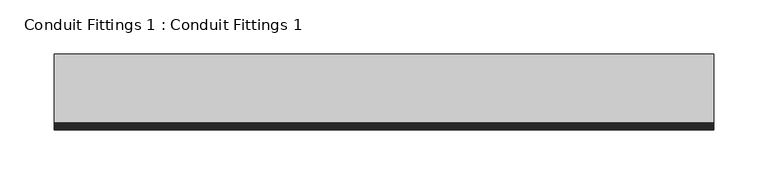
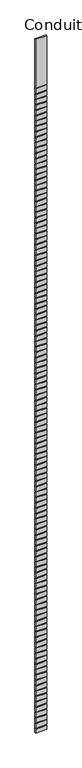
"""IFC4 building model written with IfcOpenShell, lengths in millimetres: cable carrier fitting geometry, Conduit Fittings 1 : Conduit Fittings 1."""

from ifc_helpers import new_model, si_unit, frame, origin, place, context, project, spatial, polyline, outline, extrude, source, transform, mapped, element, save


def conduit_fittings_1_conduit_fittings_1_d54f14cf(model_context):
    return source(origin(), model_context, "Body", "SweptSolid", [
        extrude(outline(polyline([(-5870.497125, -371.2934478), (-6480.097125, -371.2934478), (-6480.097125, -307.7934478), (-5870.497125, -307.7934478), (-5870.497125, -371.2934478)])), frame((0.0, 0.0, 2946.4), z_axis=(0.0, 0.0, 1.0), x_axis=(1.0, 0.0, 0.0)), (0.0, 0.0, 1.0), 225.4745322),
        extrude(outline(polyline([(-5870.497125, -371.2934478), (-6480.097125, -371.2934478), (-6480.097125, -307.7934478), (-5870.497125, -307.7934478), (-5870.497125, -371.2934478)])), frame((0.0, 0.0, 39493.8745322), z_axis=(0.0, 0.0, 1.0), x_axis=(1.0, 0.0, 0.0)), (0.0, 0.0, 1.0), 2771.7254678),
        extrude(outline(polyline([(-5870.497125, -371.2934478), (-6480.097125, -371.2934478), (-6480.097125, -307.7934478), (-5870.497125, -307.7934478), (-5870.497125, -371.2934478)])), frame((0.0, 0.0, 3222.6745322), z_axis=(0.0, 0.0, 1.0), x_axis=(1.0, 0.0, 0.0)), (0.0, 0.0, 1.0), 254.0),
        extrude(outline(polyline([(-5870.497125, -371.2934478), (-6480.097125, -371.2934478), (-6480.097125, -307.7934478), (-5870.497125, -307.7934478), (-5870.497125, -371.2934478)])), frame((0.0, 0.0, 3527.4745322), z_axis=(0.0, 0.0, 1.0), x_axis=(1.0, 0.0, 0.0)), (0.0, 0.0, 1.0), 254.0),
        extrude(outline(polyline([(-5870.497125, -371.2934478), (-6480.097125, -371.2934478), (-6480.097125, -307.7934478), (-5870.497125, -307.7934478), (-5870.497125, -371.2934478)])), frame((0.0, 0.0, 3832.2745322), z_axis=(0.0, 0.0, 1.0), x_axis=(1.0, 0.0, 0.0)), (0.0, 0.0, 1.0), 254.0),
        extrude(outline(polyline([(-5870.497125, -371.2934478), (-6480.097125, -371.2934478), (-6480.097125, -307.7934478), (-5870.497125, -307.7934478), (-5870.497125, -371.2934478)])), frame((0.0, 0.0, 4137.0745322), z_axis=(0.0, 0.0, 1.0), x_axis=(1.0, 0.0, 0.0)), (0.0, 0.0, 1.0), 254.0),
        extrude(outline(polyline([(-5870.497125, -371.2934478), (-6480.097125, -371.2934478), (-6480.097125, -307.7934478), (-5870.497125, -307.7934478), (-5870.497125, -371.2934478)])), frame((0.0, 0.0, 4441.8745322), z_axis=(0.0, 0.0, 1.0), x_axis=(1.0, 0.0, 0.0)), (0.0, 0.0, 1.0), 254.0),
        extrude(outline(polyline([(-5870.497125, -371.2934478), (-6480.097125, -371.2934478), (-6480.097125, -307.7934478), (-5870.497125, -307.7934478), (-5870.497125, -371.2934478)])), frame((0.0, 0.0, 4746.6745322), z_axis=(0.0, 0.0, 1.0), x_axis=(1.0, 0.0, 0.0)), (0.0, 0.0, 1.0), 254.0),
        extrude(outline(polyline([(-5870.497125, -371.2934478), (-6480.097125, -371.2934478), (-6480.097125, -307.7934478), (-5870.497125, -307.7934478), (-5870.497125, -371.2934478)])), frame((0.0, 0.0, 5051.4745322), z_axis=(0.0, 0.0, 1.0), x_axis=(1.0, 0.0, 0.0)), (0.0, 0.0, 1.0), 254.0),
        extrude(outline(polyline([(-5870.497125, -371.2934478), (-6480.097125, -371.2934478), (-6480.097125, -307.7934478), (-5870.497125, -307.7934478), (-5870.497125, -371.2934478)])), frame((0.0, 0.0, 5356.2745322), z_axis=(0.0, 0.0, 1.0), x_axis=(1.0, 0.0, 0.0)), (0.0, 0.0, 1.0), 254.0),
        extrude(outline(polyline([(-5870.497125, -371.2934478), (-6480.097125, -371.2934478), (-6480.097125, -307.7934478), (-5870.497125, -307.7934478), (-5870.497125, -371.2934478)])), frame((0.0, 0.0, 5661.0745322), z_axis=(0.0, 0.0, 1.0), x_axis=(1.0, 0.0, 0.0)), (0.0, 0.0, 1.0), 254.0),
        extrude(outline(polyline([(-5870.497125, -371.2934478), (-6480.097125, -371.2934478), (-6480.097125, -307.7934478), (-5870.497125, -307.7934478), (-5870.497125, -371.2934478)])), frame((0.0, 0.0, 5965.8745322), z_axis=(0.0, 0.0, 1.0), x_axis=(1.0, 0.0, 0.0)), (0.0, 0.0, 1.0), 254.0),
        extrude(outline(polyline([(-5870.497125, -371.2934478), (-6480.097125, -371.2934478), (-6480.097125, -307.7934478), (-5870.497125, -307.7934478), (-5870.497125, -371.2934478)])), frame((0.0, 0.0, 6270.6745322), z_axis=(0.0, 0.0, 1.0), x_axis=(1.0, 0.0, 0.0)), (0.0, 0.0, 1.0), 254.0),
        extrude(outline(polyline([(-5870.497125, -371.2934478), (-6480.097125, -371.2934478), (-6480.097125, -307.7934478), (-5870.497125, -307.7934478), (-5870.497125, -371.2934478)])), frame((0.0, 0.0, 6575.4745322), z_axis=(0.0, 0.0, 1.0), x_axis=(1.0, 0.0, 0.0)), (0.0, 0.0, 1.0), 254.0),
        extrude(outline(polyline([(-5870.497125, -371.2934478), (-6480.097125, -371.2934478), (-6480.097125, -307.7934478), (-5870.497125, -307.7934478), (-5870.497125, -371.2934478)])), frame((0.0, 0.0, 6880.2745322), z_axis=(0.0, 0.0, 1.0), x_axis=(1.0, 0.0, 0.0)), (0.0, 0.0, 1.0), 254.0),
        extrude(outline(polyline([(-5870.497125, -371.2934478), (-6480.097125, -371.2934478), (-6480.097125, -307.7934478), (-5870.497125, -307.7934478), (-5870.497125, -371.2934478)])), frame((0.0, 0.0, 7185.0745322), z_axis=(0.0, 0.0, 1.0), x_axis=(1.0, 0.0, 0.0)), (0.0, 0.0, 1.0), 254.0),
        extrude(outline(polyline([(-5870.497125, -371.2934478), (-6480.097125, -371.2934478), (-6480.097125, -307.7934478), (-5870.497125, -307.7934478), (-5870.497125, -371.2934478)])), frame((0.0, 0.0, 7489.8745322), z_axis=(0.0, 0.0, 1.0), x_axis=(1.0, 0.0, 0.0)), (0.0, 0.0, 1.0), 254.0),
        extrude(outline(polyline([(-5870.497125, -371.2934478), (-6480.097125, -371.2934478), (-6480.097125, -307.7934478), (-5870.497125, -307.7934478), (-5870.497125, -371.2934478)])), frame((0.0, 0.0, 7794.6745322), z_axis=(0.0, 0.0, 1.0), x_axis=(1.0, 0.0, 0.0)), (0.0, 0.0, 1.0), 254.0),
        extrude(outline(polyline([(-5870.497125, -371.2934478), (-6480.097125, -371.2934478), (-6480.097125, -307.7934478), (-5870.497125, -307.7934478), (-5870.497125, -371.2934478)])), frame((0.0, 0.0, 8099.4745322), z_axis=(0.0, 0.0, 1.0), x_axis=(1.0, 0.0, 0.0)), (0.0, 0.0, 1.0), 254.0),
        extrude(outline(polyline([(-5870.497125, -371.2934478), (-6480.097125, -371.2934478), (-6480.097125, -307.7934478), (-5870.497125, -307.7934478), (-5870.497125, -371.2934478)])), frame((0.0, 0.0, 8404.2745322), z_axis=(0.0, 0.0, 1.0), x_axis=(1.0, 0.0, 0.0)), (0.0, 0.0, 1.0), 254.0),
        extrude(outline(polyline([(-5870.497125, -371.2934478), (-6480.097125, -371.2934478), (-6480.097125, -307.7934478), (-5870.497125, -307.7934478), (-5870.497125, -371.2934478)])), frame((0.0, 0.0, 8709.0745322), z_axis=(0.0, 0.0, 1.0), x_axis=(1.0, 0.0, 0.0)), (0.0, 0.0, 1.0), 254.0),
        extrude(outline(polyline([(-5870.497125, -371.2934478), (-6480.097125, -371.2934478), (-6480.097125, -307.7934478), (-5870.497125, -307.7934478), (-5870.497125, -371.2934478)])), frame((0.0, 0.0, 9013.8745322), z_axis=(0.0, 0.0, 1.0), x_axis=(1.0, 0.0, 0.0)), (0.0, 0.0, 1.0), 254.0),
        extrude(outline(polyline([(-5870.497125, -371.2934478), (-6480.097125, -371.2934478), (-6480.097125, -307.7934478), (-5870.497125, -307.7934478), (-5870.497125, -371.2934478)])), frame((0.0, 0.0, 9318.6745322), z_axis=(0.0, 0.0, 1.0), x_axis=(1.0, 0.0, 0.0)), (0.0, 0.0, 1.0), 254.0),
        extrude(outline(polyline([(-5870.497125, -371.2934478), (-6480.097125, -371.2934478), (-6480.097125, -307.7934478), (-5870.497125, -307.7934478), (-5870.497125, -371.2934478)])), frame((0.0, 0.0, 9623.4745322), z_axis=(0.0, 0.0, 1.0), x_axis=(1.0, 0.0, 0.0)), (0.0, 0.0, 1.0), 254.0),
        extrude(outline(polyline([(-5870.497125, -371.2934478), (-6480.097125, -371.2934478), (-6480.097125, -307.7934478), (-5870.497125, -307.7934478), (-5870.497125, -371.2934478)])), frame((0.0, 0.0, 9928.2745322), z_axis=(0.0, 0.0, 1.0), x_axis=(1.0, 0.0, 0.0)), (0.0, 0.0, 1.0), 254.0),
        extrude(outline(polyline([(-5870.497125, -371.2934478), (-6480.097125, -371.2934478), (-6480.097125, -307.7934478), (-5870.497125, -307.7934478), (-5870.497125, -371.2934478)])), frame((0.0, 0.0, 10233.0745322), z_axis=(0.0, 0.0, 1.0), x_axis=(1.0, 0.0, 0.0)), (0.0, 0.0, 1.0), 254.0),
        extrude(outline(polyline([(-5870.497125, -371.2934478), (-6480.097125, -371.2934478), (-6480.097125, -307.7934478), (-5870.497125, -307.7934478), (-5870.497125, -371.2934478)])), frame((0.0, 0.0, 10537.8745322), z_axis=(0.0, 0.0, 1.0), x_axis=(1.0, 0.0, 0.0)), (0.0, 0.0, 1.0), 254.0),
        extrude(outline(polyline([(-5870.497125, -371.2934478), (-6480.097125, -371.2934478), (-6480.097125, -307.7934478), (-5870.497125, -307.7934478), (-5870.497125, -371.2934478)])), frame((0.0, 0.0, 10842.6745322), z_axis=(0.0, 0.0, 1.0), x_axis=(1.0, 0.0, 0.0)), (0.0, 0.0, 1.0), 254.0),
        extrude(outline(polyline([(-5870.497125, -371.2934478), (-6480.097125, -371.2934478), (-6480.097125, -307.7934478), (-5870.497125, -307.7934478), (-5870.497125, -371.2934478)])), frame((0.0, 0.0, 11147.4745322), z_axis=(0.0, 0.0, 1.0), x_axis=(1.0, 0.0, 0.0)), (0.0, 0.0, 1.0), 254.0),
        extrude(outline(polyline([(-5870.497125, -371.2934478), (-6480.097125, -371.2934478), (-6480.097125, -307.7934478), (-5870.497125, -307.7934478), (-5870.497125, -371.2934478)])), frame((0.0, 0.0, 11452.2745322), z_axis=(0.0, 0.0, 1.0), x_axis=(1.0, 0.0, 0.0)), (0.0, 0.0, 1.0), 254.0),
        extrude(outline(polyline([(-5870.497125, -371.2934478), (-6480.097125, -371.2934478), (-6480.097125, -307.7934478), (-5870.497125, -307.7934478), (-5870.497125, -371.2934478)])), frame((0.0, 0.0, 11757.0745322), z_axis=(0.0, 0.0, 1.0), x_axis=(1.0, 0.0, 0.0)), (0.0, 0.0, 1.0), 254.0),
        extrude(outline(polyline([(-5870.497125, -371.2934478), (-6480.097125, -371.2934478), (-6480.097125, -307.7934478), (-5870.497125, -307.7934478), (-5870.497125, -371.2934478)])), frame((0.0, 0.0, 12061.8745322), z_axis=(0.0, 0.0, 1.0), x_axis=(1.0, 0.0, 0.0)), (0.0, 0.0, 1.0), 254.0),
        extrude(outline(polyline([(-5870.497125, -371.2934478), (-6480.097125, -371.2934478), (-6480.097125, -307.7934478), (-5870.497125, -307.7934478), (-5870.497125, -371.2934478)])), frame((0.0, 0.0, 12366.6745322), z_axis=(0.0, 0.0, 1.0), x_axis=(1.0, 0.0, 0.0)), (0.0, 0.0, 1.0), 254.0),
        extrude(outline(polyline([(-5870.497125, -371.2934478), (-6480.097125, -371.2934478), (-6480.097125, -307.7934478), (-5870.497125, -307.7934478), (-5870.497125, -371.2934478)])), frame((0.0, 0.0, 12671.4745322), z_axis=(0.0, 0.0, 1.0), x_axis=(1.0, 0.0, 0.0)), (0.0, 0.0, 1.0), 254.0),
        extrude(outline(polyline([(-5870.497125, -371.2934478), (-6480.097125, -371.2934478), (-6480.097125, -307.7934478), (-5870.497125, -307.7934478), (-5870.497125, -371.2934478)])), frame((0.0, 0.0, 12976.2745322), z_axis=(0.0, 0.0, 1.0), x_axis=(1.0, 0.0, 0.0)), (0.0, 0.0, 1.0), 254.0),
        extrude(outline(polyline([(-5870.497125, -371.2934478), (-6480.097125, -371.2934478), (-6480.097125, -307.7934478), (-5870.497125, -307.7934478), (-5870.497125, -371.2934478)])), frame((0.0, 0.0, 13281.0745322), z_axis=(0.0, 0.0, 1.0), x_axis=(1.0, 0.0, 0.0)), (0.0, 0.0, 1.0), 254.0),
        extrude(outline(polyline([(-5870.497125, -371.2934478), (-6480.097125, -371.2934478), (-6480.097125, -307.7934478), (-5870.497125, -307.7934478), (-5870.497125, -371.2934478)])), frame((0.0, 0.0, 13585.8745322), z_axis=(0.0, 0.0, 1.0), x_axis=(1.0, 0.0, 0.0)), (0.0, 0.0, 1.0), 254.0),
        extrude(outline(polyline([(-5870.497125, -371.2934478), (-6480.097125, -371.2934478), (-6480.097125, -307.7934478), (-5870.497125, -307.7934478), (-5870.497125, -371.2934478)])), frame((0.0, 0.0, 13890.6745322), z_axis=(0.0, 0.0, 1.0), x_axis=(1.0, 0.0, 0.0)), (0.0, 0.0, 1.0), 254.0),
        extrude(outline(polyline([(-5870.497125, -371.2934478), (-6480.097125, -371.2934478), (-6480.097125, -307.7934478), (-5870.497125, -307.7934478), (-5870.497125, -371.2934478)])), frame((0.0, 0.0, 14195.4745322), z_axis=(0.0, 0.0, 1.0), x_axis=(1.0, 0.0, 0.0)), (0.0, 0.0, 1.0), 254.0),
        extrude(outline(polyline([(-5870.497125, -371.2934478), (-6480.097125, -371.2934478), (-6480.097125, -307.7934478), (-5870.497125, -307.7934478), (-5870.497125, -371.2934478)])), frame((0.0, 0.0, 14500.2745322), z_axis=(0.0, 0.0, 1.0), x_axis=(1.0, 0.0, 0.0)), (0.0, 0.0, 1.0), 254.0),
        extrude(outline(polyline([(-5870.497125, -371.2934478), (-6480.097125, -371.2934478), (-6480.097125, -307.7934478), (-5870.497125, -307.7934478), (-5870.497125, -371.2934478)])), frame((0.0, 0.0, 14805.0745322), z_axis=(0.0, 0.0, 1.0), x_axis=(1.0, 0.0, 0.0)), (0.0, 0.0, 1.0), 254.0),
        extrude(outline(polyline([(-5870.497125, -371.2934478), (-6480.097125, -371.2934478), (-6480.097125, -307.7934478), (-5870.497125, -307.7934478), (-5870.497125, -371.2934478)])), frame((0.0, 0.0, 15109.8745322), z_axis=(0.0, 0.0, 1.0), x_axis=(1.0, 0.0, 0.0)), (0.0, 0.0, 1.0), 254.0),
        extrude(outline(polyline([(-5870.497125, -371.2934478), (-6480.097125, -371.2934478), (-6480.097125, -307.7934478), (-5870.497125, -307.7934478), (-5870.497125, -371.2934478)])), frame((0.0, 0.0, 15414.6745322), z_axis=(0.0, 0.0, 1.0), x_axis=(1.0, 0.0, 0.0)), (0.0, 0.0, 1.0), 254.0),
        extrude(outline(polyline([(-5870.497125, -371.2934478), (-6480.097125, -371.2934478), (-6480.097125, -307.7934478), (-5870.497125, -307.7934478), (-5870.497125, -371.2934478)])), frame((0.0, 0.0, 15719.4745322), z_axis=(0.0, 0.0, 1.0), x_axis=(1.0, 0.0, 0.0)), (0.0, 0.0, 1.0), 254.0),
        extrude(outline(polyline([(-5870.497125, -371.2934478), (-6480.097125, -371.2934478), (-6480.097125, -307.7934478), (-5870.497125, -307.7934478), (-5870.497125, -371.2934478)])), frame((0.0, 0.0, 16024.2745322), z_axis=(0.0, 0.0, 1.0), x_axis=(1.0, 0.0, 0.0)), (0.0, 0.0, 1.0), 254.0),
        extrude(outline(polyline([(-5870.497125, -371.2934478), (-6480.097125, -371.2934478), (-6480.097125, -307.7934478), (-5870.497125, -307.7934478), (-5870.497125, -371.2934478)])), frame((0.0, 0.0, 16329.0745322), z_axis=(0.0, 0.0, 1.0), x_axis=(1.0, 0.0, 0.0)), (0.0, 0.0, 1.0), 254.0),
        extrude(outline(polyline([(-5870.497125, -371.2934478), (-6480.097125, -371.2934478), (-6480.097125, -307.7934478), (-5870.497125, -307.7934478), (-5870.497125, -371.2934478)])), frame((0.0, 0.0, 16633.8745322), z_axis=(0.0, 0.0, 1.0), x_axis=(1.0, 0.0, 0.0)), (0.0, 0.0, 1.0), 254.0),
        extrude(outline(polyline([(-5870.497125, -371.2934478), (-6480.097125, -371.2934478), (-6480.097125, -307.7934478), (-5870.497125, -307.7934478), (-5870.497125, -371.2934478)])), frame((0.0, 0.0, 16938.6745322), z_axis=(0.0, 0.0, 1.0), x_axis=(1.0, 0.0, 0.0)), (0.0, 0.0, 1.0), 254.0),
        extrude(outline(polyline([(-5870.497125, -371.2934478), (-6480.097125, -371.2934478), (-6480.097125, -307.7934478), (-5870.497125, -307.7934478), (-5870.497125, -371.2934478)])), frame((0.0, 0.0, 17243.4745322), z_axis=(0.0, 0.0, 1.0), x_axis=(1.0, 0.0, 0.0)), (0.0, 0.0, 1.0), 254.0),
        extrude(outline(polyline([(-5870.497125, -371.2934478), (-6480.097125, -371.2934478), (-6480.097125, -307.7934478), (-5870.497125, -307.7934478), (-5870.497125, -371.2934478)])), frame((0.0, 0.0, 17548.2745322), z_axis=(0.0, 0.0, 1.0), x_axis=(1.0, 0.0, 0.0)), (0.0, 0.0, 1.0), 254.0),
        extrude(outline(polyline([(-5870.497125, -371.2934478), (-6480.097125, -371.2934478), (-6480.097125, -307.7934478), (-5870.497125, -307.7934478), (-5870.497125, -371.2934478)])), frame((0.0, 0.0, 17853.0745322), z_axis=(0.0, 0.0, 1.0), x_axis=(1.0, 0.0, 0.0)), (0.0, 0.0, 1.0), 254.0),
        extrude(outline(polyline([(-5870.497125, -371.2934478), (-6480.097125, -371.2934478), (-6480.097125, -307.7934478), (-5870.497125, -307.7934478), (-5870.497125, -371.2934478)])), frame((0.0, 0.0, 18157.8745322), z_axis=(0.0, 0.0, 1.0), x_axis=(1.0, 0.0, 0.0)), (0.0, 0.0, 1.0), 254.0),
        extrude(outline(polyline([(-5870.497125, -371.2934478), (-6480.097125, -371.2934478), (-6480.097125, -307.7934478), (-5870.497125, -307.7934478), (-5870.497125, -371.2934478)])), frame((0.0, 0.0, 18462.6745322), z_axis=(0.0, 0.0, 1.0), x_axis=(1.0, 0.0, 0.0)), (0.0, 0.0, 1.0), 254.0),
        extrude(outline(polyline([(-5870.497125, -371.2934478), (-6480.097125, -371.2934478), (-6480.097125, -307.7934478), (-5870.497125, -307.7934478), (-5870.497125, -371.2934478)])), frame((0.0, 0.0, 18767.4745322), z_axis=(0.0, 0.0, 1.0), x_axis=(1.0, 0.0, 0.0)), (0.0, 0.0, 1.0), 254.0),
        extrude(outline(polyline([(-5870.497125, -371.2934478), (-6480.097125, -371.2934478), (-6480.097125, -307.7934478), (-5870.497125, -307.7934478), (-5870.497125, -371.2934478)])), frame((0.0, 0.0, 19072.2745322), z_axis=(0.0, 0.0, 1.0), x_axis=(1.0, 0.0, 0.0)), (0.0, 0.0, 1.0), 254.0),
        extrude(outline(polyline([(-5870.497125, -371.2934478), (-6480.097125, -371.2934478), (-6480.097125, -307.7934478), (-5870.497125, -307.7934478), (-5870.497125, -371.2934478)])), frame((0.0, 0.0, 19377.0745322), z_axis=(0.0, 0.0, 1.0), x_axis=(1.0, 0.0, 0.0)), (0.0, 0.0, 1.0), 254.0),
        extrude(outline(polyline([(-5870.497125, -371.2934478), (-6480.097125, -371.2934478), (-6480.097125, -307.7934478), (-5870.497125, -307.7934478), (-5870.497125, -371.2934478)])), frame((0.0, 0.0, 19681.8745322), z_axis=(0.0, 0.0, 1.0), x_axis=(1.0, 0.0, 0.0)), (0.0, 0.0, 1.0), 254.0),
        extrude(outline(polyline([(-5870.497125, -371.2934478), (-6480.097125, -371.2934478), (-6480.097125, -307.7934478), (-5870.497125, -307.7934478), (-5870.497125, -371.2934478)])), frame((0.0, 0.0, 19986.6745322), z_axis=(0.0, 0.0, 1.0), x_axis=(1.0, 0.0, 0.0)), (0.0, 0.0, 1.0), 254.0),
        extrude(outline(polyline([(-5870.497125, -371.2934478), (-6480.097125, -371.2934478), (-6480.097125, -307.7934478), (-5870.497125, -307.7934478), (-5870.497125, -371.2934478)])), frame((0.0, 0.0, 20291.4745322), z_axis=(0.0, 0.0, 1.0), x_axis=(1.0, 0.0, 0.0)), (0.0, 0.0, 1.0), 254.0),
        extrude(outline(polyline([(-5870.497125, -371.2934478), (-6480.097125, -371.2934478), (-6480.097125, -307.7934478), (-5870.497125, -307.7934478), (-5870.497125, -371.2934478)])), frame((0.0, 0.0, 20596.2745322), z_axis=(0.0, 0.0, 1.0), x_axis=(1.0, 0.0, 0.0)), (0.0, 0.0, 1.0), 254.0),
        extrude(outline(polyline([(-5870.497125, -371.2934478), (-6480.097125, -371.2934478), (-6480.097125, -307.7934478), (-5870.497125, -307.7934478), (-5870.497125, -371.2934478)])), frame((0.0, 0.0, 20901.0745322), z_axis=(0.0, 0.0, 1.0), x_axis=(1.0, 0.0, 0.0)), (0.0, 0.0, 1.0), 254.0),
        extrude(outline(polyline([(-5870.497125, -371.2934478), (-6480.097125, -371.2934478), (-6480.097125, -307.7934478), (-5870.497125, -307.7934478), (-5870.497125, -371.2934478)])), frame((0.0, 0.0, 21205.8745322), z_axis=(0.0, 0.0, 1.0), x_axis=(1.0, 0.0, 0.0)), (0.0, 0.0, 1.0), 254.0),
        extrude(outline(polyline([(-5870.497125, -371.2934478), (-6480.097125, -371.2934478), (-6480.097125, -307.7934478), (-5870.497125, -307.7934478), (-5870.497125, -371.2934478)])), frame((0.0, 0.0, 21510.6745322), z_axis=(0.0, 0.0, 1.0), x_axis=(1.0, 0.0, 0.0)), (0.0, 0.0, 1.0), 254.0),
        extrude(outline(polyline([(-5870.497125, -371.2934478), (-6480.097125, -371.2934478), (-6480.097125, -307.7934478), (-5870.497125, -307.7934478), (-5870.497125, -371.2934478)])), frame((0.0, 0.0, 21815.4745322), z_axis=(0.0, 0.0, 1.0), x_axis=(1.0, 0.0, 0.0)), (0.0, 0.0, 1.0), 254.0),
        extrude(outline(polyline([(-5870.497125, -371.2934478), (-6480.097125, -371.2934478), (-6480.097125, -307.7934478), (-5870.497125, -307.7934478), (-5870.497125, -371.2934478)])), frame((0.0, 0.0, 22120.2745322), z_axis=(0.0, 0.0, 1.0), x_axis=(1.0, 0.0, 0.0)), (0.0, 0.0, 1.0), 254.0),
        extrude(outline(polyline([(-5870.497125, -371.2934478), (-6480.097125, -371.2934478), (-6480.097125, -307.7934478), (-5870.497125, -307.7934478), (-5870.497125, -371.2934478)])), frame((0.0, 0.0, 22425.0745322), z_axis=(0.0, 0.0, 1.0), x_axis=(1.0, 0.0, 0.0)), (0.0, 0.0, 1.0), 254.0),
        extrude(outline(polyline([(-5870.497125, -371.2934478), (-6480.097125, -371.2934478), (-6480.097125, -307.7934478), (-5870.497125, -307.7934478), (-5870.497125, -371.2934478)])), frame((0.0, 0.0, 22729.8745322), z_axis=(0.0, 0.0, 1.0), x_axis=(1.0, 0.0, 0.0)), (0.0, 0.0, 1.0), 254.0),
        extrude(outline(polyline([(-5870.497125, -371.2934478), (-6480.097125, -371.2934478), (-6480.097125, -307.7934478), (-5870.497125, -307.7934478), (-5870.497125, -371.2934478)])), frame((0.0, 0.0, 23034.6745322), z_axis=(0.0, 0.0, 1.0), x_axis=(1.0, 0.0, 0.0)), (0.0, 0.0, 1.0), 254.0),
        extrude(outline(polyline([(-5870.497125, -371.2934478), (-6480.097125, -371.2934478), (-6480.097125, -307.7934478), (-5870.497125, -307.7934478), (-5870.497125, -371.2934478)])), frame((0.0, 0.0, 23339.4745322), z_axis=(0.0, 0.0, 1.0), x_axis=(1.0, 0.0, 0.0)), (0.0, 0.0, 1.0), 254.0),
        extrude(outline(polyline([(-5870.497125, -371.2934478), (-6480.097125, -371.2934478), (-6480.097125, -307.7934478), (-5870.497125, -307.7934478), (-5870.497125, -371.2934478)])), frame((0.0, 0.0, 23644.2745322), z_axis=(0.0, 0.0, 1.0), x_axis=(1.0, 0.0, 0.0)), (0.0, 0.0, 1.0), 254.0),
        extrude(outline(polyline([(-5870.497125, -371.2934478), (-6480.097125, -371.2934478), (-6480.097125, -307.7934478), (-5870.497125, -307.7934478), (-5870.497125, -371.2934478)])), frame((0.0, 0.0, 23949.0745322), z_axis=(0.0, 0.0, 1.0), x_axis=(1.0, 0.0, 0.0)), (0.0, 0.0, 1.0), 254.0),
        extrude(outline(polyline([(-5870.497125, -371.2934478), (-6480.097125, -371.2934478), (-6480.097125, -307.7934478), (-5870.497125, -307.7934478), (-5870.497125, -371.2934478)])), frame((0.0, 0.0, 24253.8745322), z_axis=(0.0, 0.0, 1.0), x_axis=(1.0, 0.0, 0.0)), (0.0, 0.0, 1.0), 254.0),
        extrude(outline(polyline([(-5870.497125, -371.2934478), (-6480.097125, -371.2934478), (-6480.097125, -307.7934478), (-5870.497125, -307.7934478), (-5870.497125, -371.2934478)])), frame((0.0, 0.0, 24558.6745322), z_axis=(0.0, 0.0, 1.0), x_axis=(1.0, 0.0, 0.0)), (0.0, 0.0, 1.0), 254.0),
        extrude(outline(polyline([(-5870.497125, -371.2934478), (-6480.097125, -371.2934478), (-6480.097125, -307.7934478), (-5870.497125, -307.7934478), (-5870.497125, -371.2934478)])), frame((0.0, 0.0, 24863.4745322), z_axis=(0.0, 0.0, 1.0), x_axis=(1.0, 0.0, 0.0)), (0.0, 0.0, 1.0), 254.0),
        extrude(outline(polyline([(-5870.497125, -371.2934478), (-6480.097125, -371.2934478), (-6480.097125, -307.7934478), (-5870.497125, -307.7934478), (-5870.497125, -371.2934478)])), frame((0.0, 0.0, 25168.2745322), z_axis=(0.0, 0.0, 1.0), x_axis=(1.0, 0.0, 0.0)), (0.0, 0.0, 1.0), 254.0),
        extrude(outline(polyline([(-5870.497125, -371.2934478), (-6480.097125, -371.2934478), (-6480.097125, -307.7934478), (-5870.497125, -307.7934478), (-5870.497125, -371.2934478)])), frame((0.0, 0.0, 25473.0745322), z_axis=(0.0, 0.0, 1.0), x_axis=(1.0, 0.0, 0.0)), (0.0, 0.0, 1.0), 254.0),
        extrude(outline(polyline([(-5870.497125, -371.2934478), (-6480.097125, -371.2934478), (-6480.097125, -307.7934478), (-5870.497125, -307.7934478), (-5870.497125, -371.2934478)])), frame((0.0, 0.0, 25777.8745322), z_axis=(0.0, 0.0, 1.0), x_axis=(1.0, 0.0, 0.0)), (0.0, 0.0, 1.0), 254.0),
        extrude(outline(polyline([(-5870.497125, -371.2934478), (-6480.097125, -371.2934478), (-6480.097125, -307.7934478), (-5870.497125, -307.7934478), (-5870.497125, -371.2934478)])), frame((0.0, 0.0, 26082.6745322), z_axis=(0.0, 0.0, 1.0), x_axis=(1.0, 0.0, 0.0)), (0.0, 0.0, 1.0), 254.0),
        extrude(outline(polyline([(-5870.497125, -371.2934478), (-6480.097125, -371.2934478), (-6480.097125, -307.7934478), (-5870.497125, -307.7934478), (-5870.497125, -371.2934478)])), frame((0.0, 0.0, 26387.4745322), z_axis=(0.0, 0.0, 1.0), x_axis=(1.0, 0.0, 0.0)), (0.0, 0.0, 1.0), 254.0),
        extrude(outline(polyline([(-5870.497125, -371.2934478), (-6480.097125, -371.2934478), (-6480.097125, -307.7934478), (-5870.497125, -307.7934478), (-5870.497125, -371.2934478)])), frame((0.0, 0.0, 26692.2745322), z_axis=(0.0, 0.0, 1.0), x_axis=(1.0, 0.0, 0.0)), (0.0, 0.0, 1.0), 254.0),
        extrude(outline(polyline([(-5870.497125, -371.2934478), (-6480.097125, -371.2934478), (-6480.097125, -307.7934478), (-5870.497125, -307.7934478), (-5870.497125, -371.2934478)])), frame((0.0, 0.0, 26997.0745322), z_axis=(0.0, 0.0, 1.0), x_axis=(1.0, 0.0, 0.0)), (0.0, 0.0, 1.0), 254.0),
        extrude(outline(polyline([(-5870.497125, -371.2934478), (-6480.097125, -371.2934478), (-6480.097125, -307.7934478), (-5870.497125, -307.7934478), (-5870.497125, -371.2934478)])), frame((0.0, 0.0, 27301.8745322), z_axis=(0.0, 0.0, 1.0), x_axis=(1.0, 0.0, 0.0)), (0.0, 0.0, 1.0), 254.0),
        extrude(outline(polyline([(-5870.497125, -371.2934478), (-6480.097125, -371.2934478), (-6480.097125, -307.7934478), (-5870.497125, -307.7934478), (-5870.497125, -371.2934478)])), frame((0.0, 0.0, 27606.6745322), z_axis=(0.0, 0.0, 1.0), x_axis=(1.0, 0.0, 0.0)), (0.0, 0.0, 1.0), 254.0),
        extrude(outline(polyline([(-5870.497125, -371.2934478), (-6480.097125, -371.2934478), (-6480.097125, -307.7934478), (-5870.497125, -307.7934478), (-5870.497125, -371.2934478)])), frame((0.0, 0.0, 27911.4745322), z_axis=(0.0, 0.0, 1.0), x_axis=(1.0, 0.0, 0.0)), (0.0, 0.0, 1.0), 254.0),
        extrude(outline(polyline([(-5870.497125, -371.2934478), (-6480.097125, -371.2934478), (-6480.097125, -307.7934478), (-5870.497125, -307.7934478), (-5870.497125, -371.2934478)])), frame((0.0, 0.0, 28216.2745322), z_axis=(0.0, 0.0, 1.0), x_axis=(1.0, 0.0, 0.0)), (0.0, 0.0, 1.0), 254.0),
        extrude(outline(polyline([(-5870.497125, -371.2934478), (-6480.097125, -371.2934478), (-6480.097125, -307.7934478), (-5870.497125, -307.7934478), (-5870.497125, -371.2934478)])), frame((0.0, 0.0, 28521.0745322), z_axis=(0.0, 0.0, 1.0), x_axis=(1.0, 0.0, 0.0)), (0.0, 0.0, 1.0), 254.0),
        extrude(outline(polyline([(-5870.497125, -371.2934478), (-6480.097125, -371.2934478), (-6480.097125, -307.7934478), (-5870.497125, -307.7934478), (-5870.497125, -371.2934478)])), frame((0.0, 0.0, 28825.8745322), z_axis=(0.0, 0.0, 1.0), x_axis=(1.0, 0.0, 0.0)), (0.0, 0.0, 1.0), 254.0),
        extrude(outline(polyline([(-5870.497125, -371.2934478), (-6480.097125, -371.2934478), (-6480.097125, -307.7934478), (-5870.497125, -307.7934478), (-5870.497125, -371.2934478)])), frame((0.0, 0.0, 29130.6745322), z_axis=(0.0, 0.0, 1.0), x_axis=(1.0, 0.0, 0.0)), (0.0, 0.0, 1.0), 254.0),
        extrude(outline(polyline([(-5870.497125, -371.2934478), (-6480.097125, -371.2934478), (-6480.097125, -307.7934478), (-5870.497125, -307.7934478), (-5870.497125, -371.2934478)])), frame((0.0, 0.0, 29435.4745322), z_axis=(0.0, 0.0, 1.0), x_axis=(1.0, 0.0, 0.0)), (0.0, 0.0, 1.0), 254.0),
        extrude(outline(polyline([(-5870.497125, -371.2934478), (-6480.097125, -371.2934478), (-6480.097125, -307.7934478), (-5870.497125, -307.7934478), (-5870.497125, -371.2934478)])), frame((0.0, 0.0, 29740.2745322), z_axis=(0.0, 0.0, 1.0), x_axis=(1.0, 0.0, 0.0)), (0.0, 0.0, 1.0), 254.0),
        extrude(outline(polyline([(-5870.497125, -371.2934478), (-6480.097125, -371.2934478), (-6480.097125, -307.7934478), (-5870.497125, -307.7934478), (-5870.497125, -371.2934478)])), frame((0.0, 0.0, 30045.0745322), z_axis=(0.0, 0.0, 1.0), x_axis=(1.0, 0.0, 0.0)), (0.0, 0.0, 1.0), 254.0),
        extrude(outline(polyline([(-5870.497125, -371.2934478), (-6480.097125, -371.2934478), (-6480.097125, -307.7934478), (-5870.497125, -307.7934478), (-5870.497125, -371.2934478)])), frame((0.0, 0.0, 30349.8745322), z_axis=(0.0, 0.0, 1.0), x_axis=(1.0, 0.0, 0.0)), (0.0, 0.0, 1.0), 254.0),
        extrude(outline(polyline([(-5870.497125, -371.2934478), (-6480.097125, -371.2934478), (-6480.097125, -307.7934478), (-5870.497125, -307.7934478), (-5870.497125, -371.2934478)])), frame((0.0, 0.0, 30654.6745322), z_axis=(0.0, 0.0, 1.0), x_axis=(1.0, 0.0, 0.0)), (0.0, 0.0, 1.0), 254.0),
        extrude(outline(polyline([(-5870.497125, -371.2934478), (-6480.097125, -371.2934478), (-6480.097125, -307.7934478), (-5870.497125, -307.7934478), (-5870.497125, -371.2934478)])), frame((0.0, 0.0, 30959.4745322), z_axis=(0.0, 0.0, 1.0), x_axis=(1.0, 0.0, 0.0)), (0.0, 0.0, 1.0), 254.0),
        extrude(outline(polyline([(-5870.497125, -371.2934478), (-6480.097125, -371.2934478), (-6480.097125, -307.7934478), (-5870.497125, -307.7934478), (-5870.497125, -371.2934478)])), frame((0.0, 0.0, 31264.2745322), z_axis=(0.0, 0.0, 1.0), x_axis=(1.0, 0.0, 0.0)), (0.0, 0.0, 1.0), 254.0),
        extrude(outline(polyline([(-5870.497125, -371.2934478), (-6480.097125, -371.2934478), (-6480.097125, -307.7934478), (-5870.497125, -307.7934478), (-5870.497125, -371.2934478)])), frame((0.0, 0.0, 31569.0745322), z_axis=(0.0, 0.0, 1.0), x_axis=(1.0, 0.0, 0.0)), (0.0, 0.0, 1.0), 254.0),
        extrude(outline(polyline([(-5870.497125, -371.2934478), (-6480.097125, -371.2934478), (-6480.097125, -307.7934478), (-5870.497125, -307.7934478), (-5870.497125, -371.2934478)])), frame((0.0, 0.0, 31873.8745322), z_axis=(0.0, 0.0, 1.0), x_axis=(1.0, 0.0, 0.0)), (0.0, 0.0, 1.0), 254.0),
        extrude(outline(polyline([(-5870.497125, -371.2934478), (-6480.097125, -371.2934478), (-6480.097125, -307.7934478), (-5870.497125, -307.7934478), (-5870.497125, -371.2934478)])), frame((0.0, 0.0, 32178.6745322), z_axis=(0.0, 0.0, 1.0), x_axis=(1.0, 0.0, 0.0)), (0.0, 0.0, 1.0), 254.0),
        extrude(outline(polyline([(-5870.497125, -371.2934478), (-6480.097125, -371.2934478), (-6480.097125, -307.7934478), (-5870.497125, -307.7934478), (-5870.497125, -371.2934478)])), frame((0.0, 0.0, 32483.4745322), z_axis=(0.0, 0.0, 1.0), x_axis=(1.0, 0.0, 0.0)), (0.0, 0.0, 1.0), 254.0),
        extrude(outline(polyline([(-5870.497125, -371.2934478), (-6480.097125, -371.2934478), (-6480.097125, -307.7934478), (-5870.497125, -307.7934478), (-5870.497125, -371.2934478)])), frame((0.0, 0.0, 32788.2745322), z_axis=(0.0, 0.0, 1.0), x_axis=(1.0, 0.0, 0.0)), (0.0, 0.0, 1.0), 254.0),
        extrude(outline(polyline([(-5870.497125, -371.2934478), (-6480.097125, -371.2934478), (-6480.097125, -307.7934478), (-5870.497125, -307.7934478), (-5870.497125, -371.2934478)])), frame((0.0, 0.0, 33093.0745322), z_axis=(0.0, 0.0, 1.0), x_axis=(1.0, 0.0, 0.0)), (0.0, 0.0, 1.0), 254.0),
        extrude(outline(polyline([(-5870.497125, -371.2934478), (-6480.097125, -371.2934478), (-6480.097125, -307.7934478), (-5870.497125, -307.7934478), (-5870.497125, -371.2934478)])), frame((0.0, 0.0, 33397.8745322), z_axis=(0.0, 0.0, 1.0), x_axis=(1.0, 0.0, 0.0)), (0.0, 0.0, 1.0), 254.0),
        extrude(outline(polyline([(-5870.497125, -371.2934478), (-6480.097125, -371.2934478), (-6480.097125, -307.7934478), (-5870.497125, -307.7934478), (-5870.497125, -371.2934478)])), frame((0.0, 0.0, 33702.6745322), z_axis=(0.0, 0.0, 1.0), x_axis=(1.0, 0.0, 0.0)), (0.0, 0.0, 1.0), 254.0),
        extrude(outline(polyline([(-5870.497125, -371.2934478), (-6480.097125, -371.2934478), (-6480.097125, -307.7934478), (-5870.497125, -307.7934478), (-5870.497125, -371.2934478)])), frame((0.0, 0.0, 34007.4745322), z_axis=(0.0, 0.0, 1.0), x_axis=(1.0, 0.0, 0.0)), (0.0, 0.0, 1.0), 254.0),
        extrude(outline(polyline([(-5870.497125, -371.2934478), (-6480.097125, -371.2934478), (-6480.097125, -307.7934478), (-5870.497125, -307.7934478), (-5870.497125, -371.2934478)])), frame((0.0, 0.0, 34312.2745322), z_axis=(0.0, 0.0, 1.0), x_axis=(1.0, 0.0, 0.0)), (0.0, 0.0, 1.0), 254.0),
        extrude(outline(polyline([(-5870.497125, -371.2934478), (-6480.097125, -371.2934478), (-6480.097125, -307.7934478), (-5870.497125, -307.7934478), (-5870.497125, -371.2934478)])), frame((0.0, 0.0, 34617.0745322), z_axis=(0.0, 0.0, 1.0), x_axis=(1.0, 0.0, 0.0)), (0.0, 0.0, 1.0), 254.0),
        extrude(outline(polyline([(-5870.497125, -371.2934478), (-6480.097125, -371.2934478), (-6480.097125, -307.7934478), (-5870.497125, -307.7934478), (-5870.497125, -371.2934478)])), frame((0.0, 0.0, 34921.8745322), z_axis=(0.0, 0.0, 1.0), x_axis=(1.0, 0.0, 0.0)), (0.0, 0.0, 1.0), 254.0),
        extrude(outline(polyline([(-5870.497125, -371.2934478), (-6480.097125, -371.2934478), (-6480.097125, -307.7934478), (-5870.497125, -307.7934478), (-5870.497125, -371.2934478)])), frame((0.0, 0.0, 35226.6745322), z_axis=(0.0, 0.0, 1.0), x_axis=(1.0, 0.0, 0.0)), (0.0, 0.0, 1.0), 254.0),
        extrude(outline(polyline([(-5870.497125, -371.2934478), (-6480.097125, -371.2934478), (-6480.097125, -307.7934478), (-5870.497125, -307.7934478), (-5870.497125, -371.2934478)])), frame((0.0, 0.0, 35531.4745322), z_axis=(0.0, 0.0, 1.0), x_axis=(1.0, 0.0, 0.0)), (0.0, 0.0, 1.0), 254.0),
        extrude(outline(polyline([(-5870.497125, -371.2934478), (-6480.097125, -371.2934478), (-6480.097125, -307.7934478), (-5870.497125, -307.7934478), (-5870.497125, -371.2934478)])), frame((0.0, 0.0, 35836.2745322), z_axis=(0.0, 0.0, 1.0), x_axis=(1.0, 0.0, 0.0)), (0.0, 0.0, 1.0), 254.0),
        extrude(outline(polyline([(-5870.497125, -371.2934478), (-6480.097125, -371.2934478), (-6480.097125, -307.7934478), (-5870.497125, -307.7934478), (-5870.497125, -371.2934478)])), frame((0.0, 0.0, 36141.0745322), z_axis=(0.0, 0.0, 1.0), x_axis=(1.0, 0.0, 0.0)), (0.0, 0.0, 1.0), 254.0),
        extrude(outline(polyline([(-5870.497125, -371.2934478), (-6480.097125, -371.2934478), (-6480.097125, -307.7934478), (-5870.497125, -307.7934478), (-5870.497125, -371.2934478)])), frame((0.0, 0.0, 36445.8745322), z_axis=(0.0, 0.0, 1.0), x_axis=(1.0, 0.0, 0.0)), (0.0, 0.0, 1.0), 254.0),
        extrude(outline(polyline([(-5870.497125, -371.2934478), (-6480.097125, -371.2934478), (-6480.097125, -307.7934478), (-5870.497125, -307.7934478), (-5870.497125, -371.2934478)])), frame((0.0, 0.0, 36750.6745322), z_axis=(0.0, 0.0, 1.0), x_axis=(1.0, 0.0, 0.0)), (0.0, 0.0, 1.0), 254.0),
        extrude(outline(polyline([(-5870.497125, -371.2934478), (-6480.097125, -371.2934478), (-6480.097125, -307.7934478), (-5870.497125, -307.7934478), (-5870.497125, -371.2934478)])), frame((0.0, 0.0, 37055.4745322), z_axis=(0.0, 0.0, 1.0), x_axis=(1.0, 0.0, 0.0)), (0.0, 0.0, 1.0), 254.0),
        extrude(outline(polyline([(-5870.497125, -371.2934478), (-6480.097125, -371.2934478), (-6480.097125, -307.7934478), (-5870.497125, -307.7934478), (-5870.497125, -371.2934478)])), frame((0.0, 0.0, 37360.2745322), z_axis=(0.0, 0.0, 1.0), x_axis=(1.0, 0.0, 0.0)), (0.0, 0.0, 1.0), 254.0),
        extrude(outline(polyline([(-5870.497125, -371.2934478), (-6480.097125, -371.2934478), (-6480.097125, -307.7934478), (-5870.497125, -307.7934478), (-5870.497125, -371.2934478)])), frame((0.0, 0.0, 37665.0745322), z_axis=(0.0, 0.0, 1.0), x_axis=(1.0, 0.0, 0.0)), (0.0, 0.0, 1.0), 254.0),
        extrude(outline(polyline([(-5870.497125, -371.2934478), (-6480.097125, -371.2934478), (-6480.097125, -307.7934478), (-5870.497125, -307.7934478), (-5870.497125, -371.2934478)])), frame((0.0, 0.0, 37969.8745322), z_axis=(0.0, 0.0, 1.0), x_axis=(1.0, 0.0, 0.0)), (0.0, 0.0, 1.0), 254.0),
        extrude(outline(polyline([(-5870.497125, -371.2934478), (-6480.097125, -371.2934478), (-6480.097125, -307.7934478), (-5870.497125, -307.7934478), (-5870.497125, -371.2934478)])), frame((0.0, 0.0, 38274.6745322), z_axis=(0.0, 0.0, 1.0), x_axis=(1.0, 0.0, 0.0)), (0.0, 0.0, 1.0), 254.0),
        extrude(outline(polyline([(-5870.497125, -371.2934478), (-6480.097125, -371.2934478), (-6480.097125, -307.7934478), (-5870.497125, -307.7934478), (-5870.497125, -371.2934478)])), frame((0.0, 0.0, 38579.4745322), z_axis=(0.0, 0.0, 1.0), x_axis=(1.0, 0.0, 0.0)), (0.0, 0.0, 1.0), 254.0),
        extrude(outline(polyline([(-5870.497125, -371.2934478), (-6480.097125, -371.2934478), (-6480.097125, -307.7934478), (-5870.497125, -307.7934478), (-5870.497125, -371.2934478)])), frame((0.0, 0.0, 38884.2745322), z_axis=(0.0, 0.0, 1.0), x_axis=(1.0, 0.0, 0.0)), (0.0, 0.0, 1.0), 254.0),
        extrude(outline(polyline([(-5870.497125, -371.2934478), (-6480.097125, -371.2934478), (-6480.097125, -307.7934478), (-5870.497125, -307.7934478), (-5870.497125, -371.2934478)])), frame((0.0, 0.0, 39189.0745322), z_axis=(0.0, 0.0, 1.0), x_axis=(1.0, 0.0, 0.0)), (0.0, 0.0, 1.0), 282.5254678),
    ])


if __name__ == "__main__":
    model = new_model("IFC4")
    model_context = context("Model", 3, world=origin())
    ifc_project = project(units=[si_unit("LENGTHUNIT", "METRE", prefix="MILLI")], contexts=[model_context])
    site = spatial("IfcSite", under=ifc_project)
    building = spatial("IfcBuilding", under=site)
    placement = place(None, origin())
    conduit_fittings_1_conduit_fittings_1_shape = conduit_fittings_1_conduit_fittings_1_d54f14cf(model_context)
    element("IfcCableCarrierFitting", 1, ObjectType="Conduit Fittings 1 : Conduit Fittings 1", at=placement, inside=building, context=model_context, shape_type="MappedRepresentation", body=[
        mapped(conduit_fittings_1_conduit_fittings_1_shape, transform((0.0, 0.0, 0.0), x_axis=(1.0, 0.0, 0.0), y_axis=(0.0, 1.0, 0.0), z_axis=(0.0, 0.0, 1.0))),
    ])
    save(model, "model.ifc")

# Revit data of these elements
# Element 1 (IfcCableCarrierFitting, "Conduit Fittings 1 : Conduit Fittings 1")
#   Materials on its faces: "yellow"
# Materials
#   "yellow": class "Generic", colour RGB 255 255 0, transparency 0, Cost = 0
